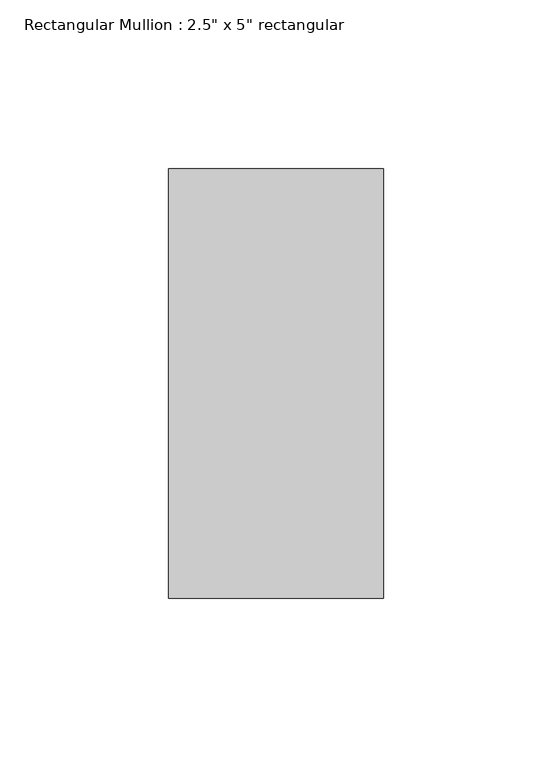
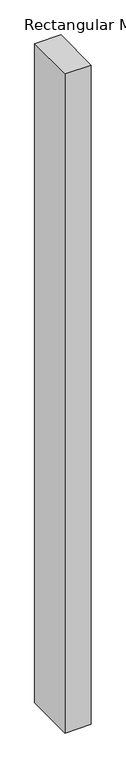
"""IFC4 building model written with IfcOpenShell, lengths in millimetres: member geometry."""

from ifc_helpers import new_model, si_unit, frame, origin, place, context, project, spatial, polyline, outline, extrude, source, transform, mapped, element, save


def member_f14600c3(model_context):
    return source(origin(), model_context, "Body", "SweptSolid", [
        extrude(outline(polyline([(31.75, 63.5), (31.75, -63.5), (-31.75, -63.5), (-31.75, 63.5), (31.75, 63.5)])), frame((0.0, 0.0, -1686.2136257), z_axis=(0.0, 0.0, 1.0), x_axis=(1.0, 0.0, 0.0)), (0.0, 0.0, 1.0), 1686.2136257),
    ])


if __name__ == "__main__":
    model = new_model("IFC4")
    model_context = context("Model", 3, world=origin())
    ifc_project = project(units=[si_unit("LENGTHUNIT", "METRE", prefix="MILLI")], contexts=[model_context])
    site = spatial("IfcSite", under=ifc_project)
    building = spatial("IfcBuilding", under=site)
    placement = place(None, origin())
    member_shape = member_f14600c3(model_context)
    element("IfcMember", 1, ObjectType="Rectangular Mullion : 2.5\" x 5\" rectangular", at=placement, inside=building, context=model_context, shape_type="MappedRepresentation", body=[
        mapped(member_shape, transform((0.0, 0.0, 0.0), x_axis=(1.0, 0.0, 0.0), y_axis=(0.0, 1.0, 0.0), z_axis=(0.0, 0.0, 1.0))),
    ])
    save(model, "model.ifc")

# Revit data of these elements
# Type "Rectangular Mullion : 2.5\" x 5\" rectangular"
#   built-in parameter 1007304 = 0.416667 (stored number, unit not read)
#   built-in parameter 1007301 = 0.104167 (stored number, unit not read)
#   built-in parameter 1007300 = 0.104167 (stored number, unit not read)
# Element 1 (IfcMember, "Rectangular Mullion : 2.5\" x 5\" rectangular")
#   Materials on its faces: "Aluminum"
# Materials
#   "Aluminum": class "Metal", colour RGB 247 247 247, transparency 0, Description = "Aluminum 6061", Cost = 0
